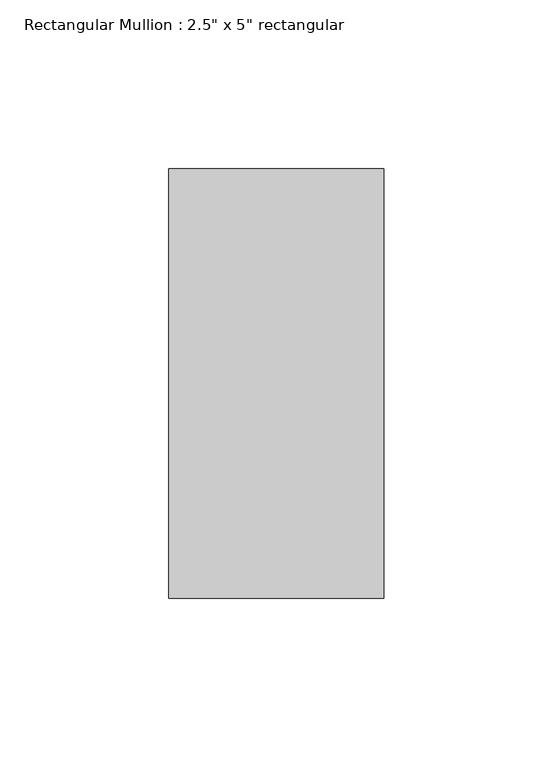
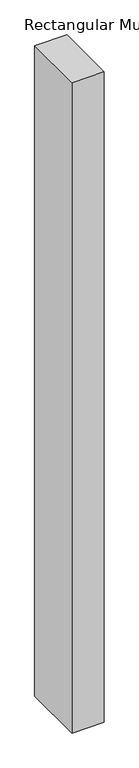
"""IFC4 building model written with IfcOpenShell, lengths in millimetres: member geometry."""

from ifc_helpers import new_model, si_unit, frame, origin, place, context, project, spatial, polyline, outline, extrude, source, transform, mapped, element, save


def member_20eb5ac3(model_context):
    return source(origin(), model_context, "Body", "SweptSolid", [
        extrude(outline(polyline([(0.0, 63.5), (0.0, -63.5), (-63.5, -63.5), (-63.5, 63.5), (0.0, 63.5)])), frame((0.0, 0.0, -1352.55), z_axis=(0.0, 0.0, 1.0), x_axis=(1.0, 0.0, 0.0)), (0.0, 0.0, 1.0), 1352.55),
    ])


if __name__ == "__main__":
    model = new_model("IFC4")
    model_context = context("Model", 3, world=origin())
    ifc_project = project(units=[si_unit("LENGTHUNIT", "METRE", prefix="MILLI")], contexts=[model_context])
    site = spatial("IfcSite", under=ifc_project)
    building = spatial("IfcBuilding", under=site)
    placement = place(None, origin())
    member_shape = member_20eb5ac3(model_context)
    element("IfcMember", 1, ObjectType="Rectangular Mullion : 2.5\" x 5\" rectangular", at=placement, inside=building, context=model_context, shape_type="MappedRepresentation", body=[
        mapped(member_shape, transform((0.0, 0.0, 0.0), x_axis=(1.0, 0.0, 0.0), y_axis=(0.0, 1.0, 0.0), z_axis=(0.0, 0.0, 1.0))),
    ])
    save(model, "model.ifc")

# Revit data of these elements
# Type "Rectangular Mullion : 2.5\" x 5\" rectangular"
#   built-in parameter 1007304 = 0.416667 (stored number, unit not read)
#   built-in parameter 1007301 = 0.104167 (stored number, unit not read)
#   built-in parameter 1007300 = 0.104167 (stored number, unit not read)
# Element 1 (IfcMember, "Rectangular Mullion : 2.5\" x 5\" rectangular")
#   Materials on its faces: "Iron, Ductile"
# Materials
#   "Iron, Ductile": class "Metal", colour RGB 0 0 0, transparency 0, Description = "Ductile cast iron", Cost = 0
